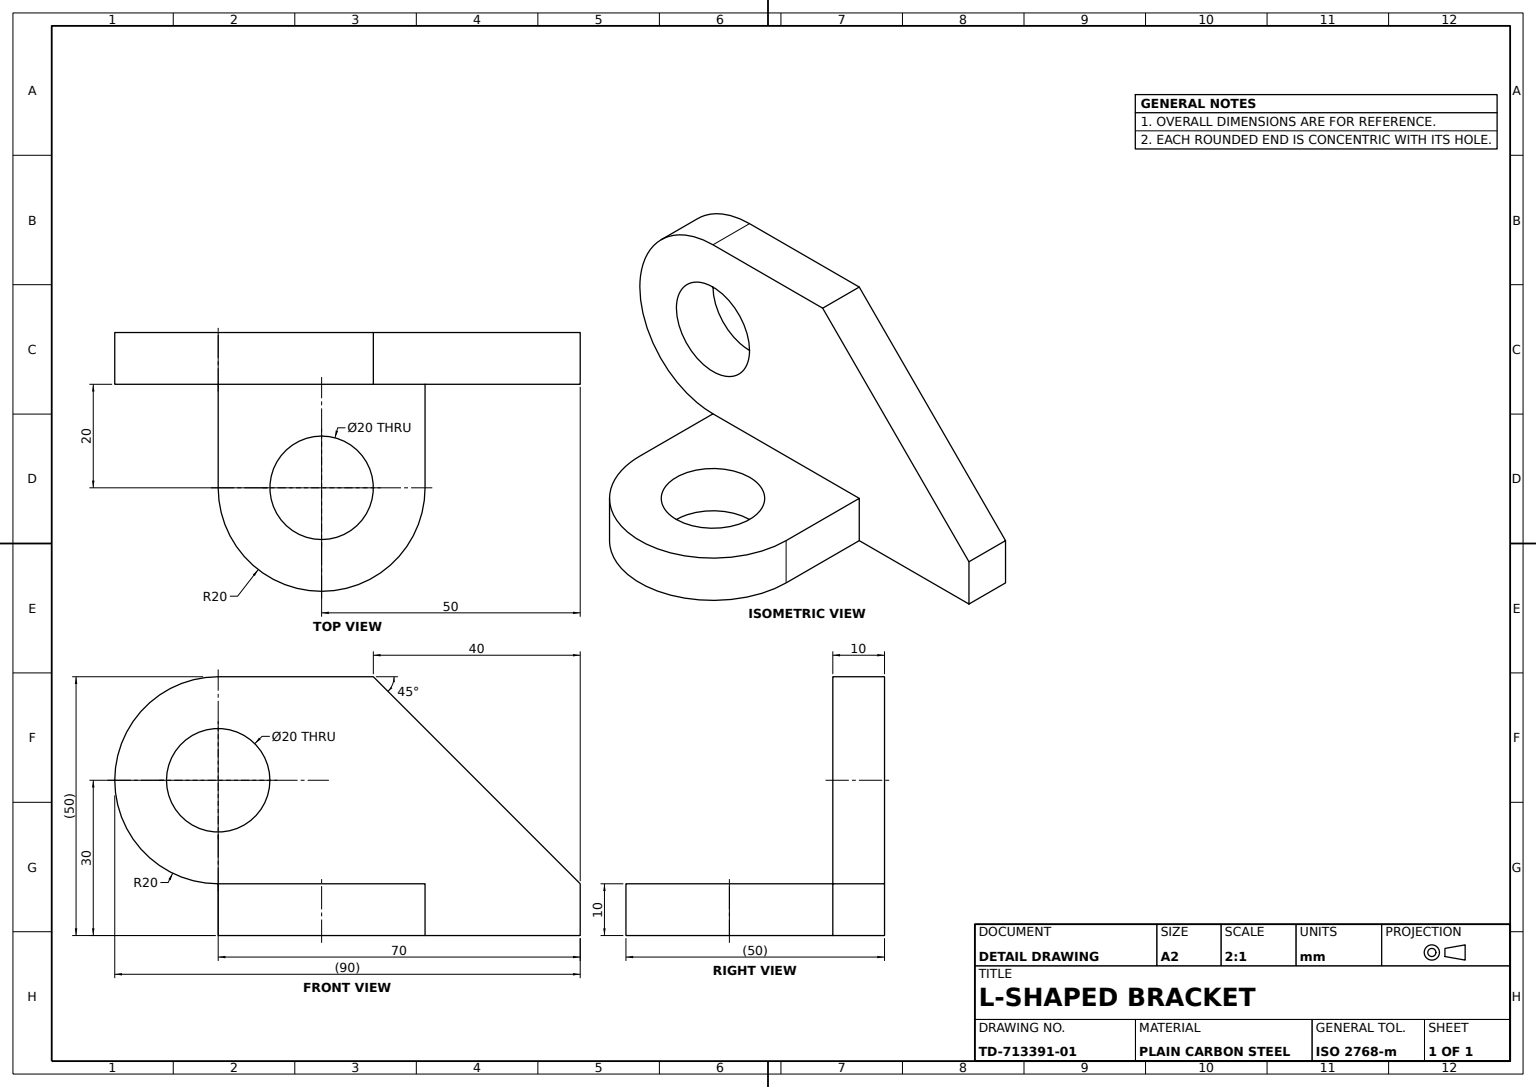
SolidWorks part; units mm, degrees
material "Plain Carbon Steel"
ref_plane "Front Plane" through (0, 0, 0) normal (0, 0, 1) x (1, 0, 0)
ref_plane "Top Plane" through (0, 0, 0) normal (0, 1, 0) x (1, 0, 0)
ref_plane "Right Plane" through (0, 0, 0) normal (1, 0, 0) x (0, 0, -1)
sketch "Upright Plate Profile" plane through (0, 0, 0) normal (0, 0, 1) x (1, 0, 0)
  line L0 (0, 50) -> (30, 50)
  line L1 (0, 0) -> (70, 0)
  line L2 (0, 0) -> (0, 10)
  line L7 (70, 0) -> (70, 10)
  line L8 (30, 50) -> (70, 10)
  arc A0 (0, 50) -> (0, 10) centre (0, 30) ccw
  point P0 (0, 0)
  dimension "D5" = 40
  dimension "D1" = 70
  dimension "D2" = 50
  dimension "D3" = 30
  dimension "D4" = 10
extrude "Upright Plate" add sketch "Upright Plate Profile" along normal mid plane 10
sketch "Base Lug Profile" plane through (0, 0, 0) normal (0, -1, 0) x (1, 0, 0)
  line L0 (0, 5) -> (70, 5) construction
  line L1 (0, 5) -> (0, 25)
  line L2 (40, 25) -> (40, 5)
  line L7 (0, -5) -> (70, -5)
  line L8 (70, -5) -> (70, 5)
  line L9 (70, 5) -> (0, 5)
  line L10 (0, 5) -> (0, -5)
  line L11 (0, -5) -> (70, -5)
  line L12 (70, -5) -> (70, 5)
  line L13 (70, 5) -> (40, 5)
  line L14 (0, 5) -> (0, -5)
  arc A1 (40, 25) -> (0, 25) centre (20, 25) ccw
  dimension "D1" = 40
  dimension "D2" = 0
extrude "Base Lug" add sketch "Base Lug Profile" against normal blind 10
sketch "Base Lug Hole Profile" plane through (0, 10, 0) normal (0, 1, 0) x (1, 0, 0)
  circle A0 centre (20, -25) radius 10
  dimension "D1" = 20
extrude "Base Lug Hole Ø20" cut sketch "Base Lug Hole Profile" against normal through all
sketch "Upright Plate Hole Profile" plane through (0, 0, 5) normal (0, 0, 1) x (1, 0, 0)
  circle A0 centre (0, 30) radius 10
  dimension "D1" = 20
extrude "Upright Plate Hole Ø20" cut sketch "Upright Plate Hole Profile" against normal through all
